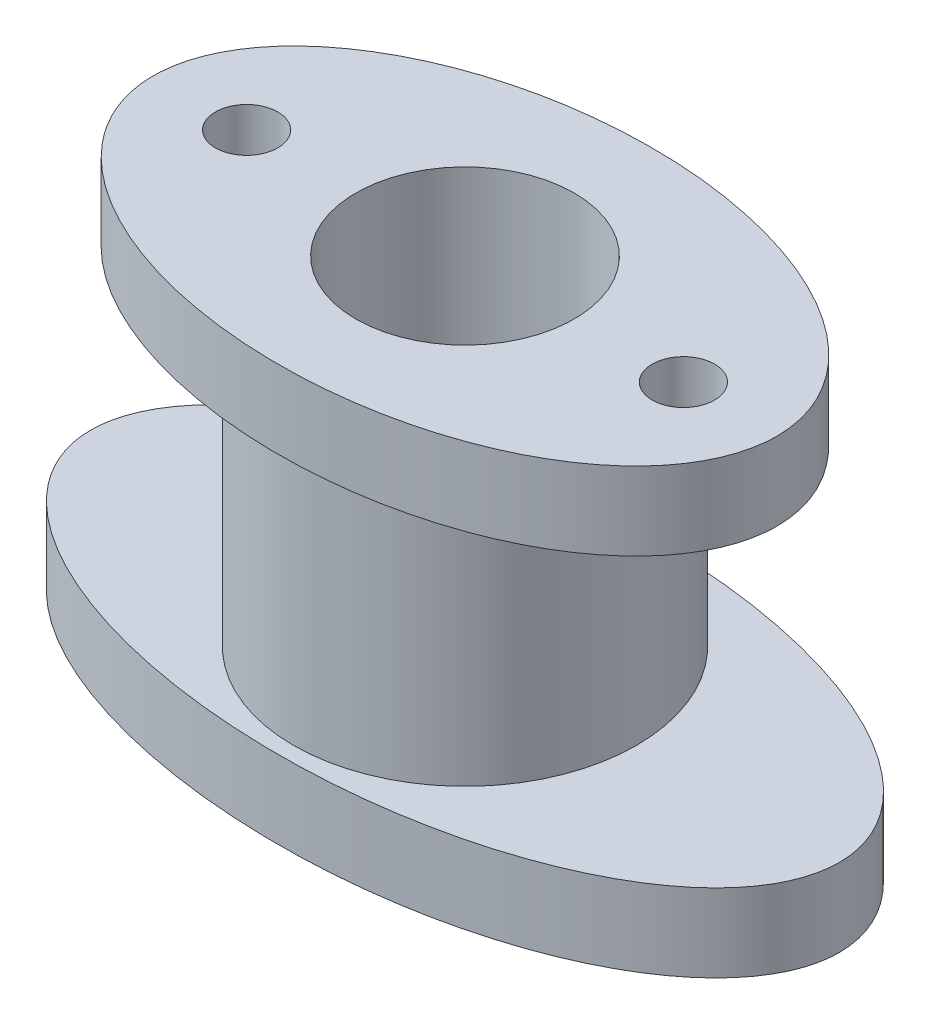
from build123d import *

# Parameters (mm, degrees)
BASE_FLANGE_SKETCH_RX             = 72
BASE_FLANGE_SKETCH_RY             = 36
BASE_FLANGE_DEPTH                 = 15
CENTER_BOSS_SKETCH_R              = 33
CENTER_BOSS_66_DEPTH              = 50
TOP_FLANGE_SKETCH_RX              = 60
TOP_FLANGE_SKETCH_RY              = 36
TOP_FLANGE_SKETCH_R               = 6
TOP_FLANGE_WITH_HOLES_2X_12_DEPTH = 15
BORE_SKETCH_R                     = 21
BORE_42_DEPTH                     = 65


with BuildPart() as part:
    # Base Flange Sketch → Base Flange (new body)
    with BuildSketch(Plane(origin=(0, 0, 0), x_dir=(1, 0, 0), z_dir=(0, 1, 0))):
        with Locations((0, 0)):
            Ellipse(BASE_FLANGE_SKETCH_RX, BASE_FLANGE_SKETCH_RY)
    extrude(amount=BASE_FLANGE_DEPTH)

    # Center Boss Sketch → Center Boss Ø66 (add)
    with BuildSketch(Plane(origin=(0, 15, 0), x_dir=(1, 0, 0), z_dir=(0, 1, 0))):
        with Locations(Location((0, 0, 0), (0, 0, 270))):
            Circle(CENTER_BOSS_SKETCH_R)
    extrude(amount=CENTER_BOSS_66_DEPTH)

    # Top Flange Sketch → Top Flange with Holes 2xØ12 (add)
    with BuildSketch(Plane(origin=(0, 65, 0), x_dir=(1, 0, 0), z_dir=(0, 1, 0))):
        with Locations((0, 0)):
            Ellipse(TOP_FLANGE_SKETCH_RX, TOP_FLANGE_SKETCH_RY)
        with Locations(Location((-42, 0, 0), (0, 0, 270))):
            Circle(TOP_FLANGE_SKETCH_R, mode=Mode.SUBTRACT)
        with Locations(Location((42, 0, 0), (0, 0, 270))):
            Circle(TOP_FLANGE_SKETCH_R, mode=Mode.SUBTRACT)
    extrude(amount=TOP_FLANGE_WITH_HOLES_2X_12_DEPTH)

    # Bore Sketch → Bore Ø42 (cut)
    with BuildSketch(Plane(origin=(0, 80, 0), x_dir=(1, 0, 0), z_dir=(0, 1, 0))):
        with Locations(Location((0, 0, 0), (0, 0, 270))):
            Circle(BORE_SKETCH_R)
    extrude(amount=-BORE_42_DEPTH, mode=Mode.SUBTRACT)


solid = part.part
